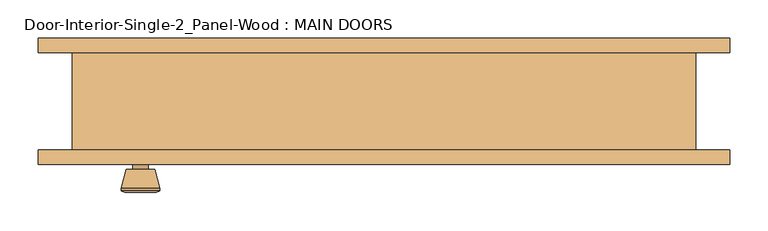
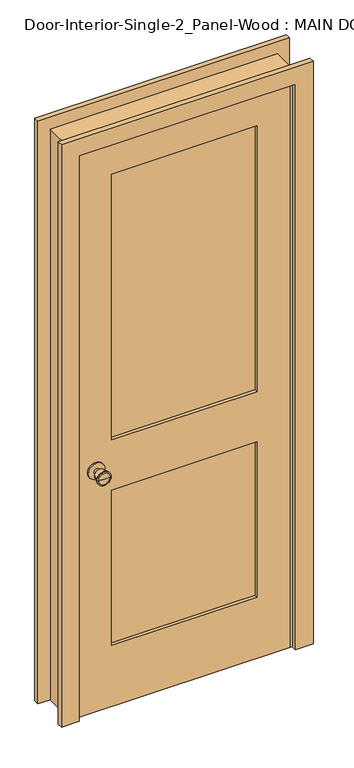
"""IFC4 building model written with IfcOpenShell, lengths in millimetres: door geometry, Door-Interior-Single-2_Panel-Wood : MAIN DOORS."""

from ifc_helpers import new_model, si_unit, point, frame, frame_2d, origin, place, context, project, spatial, polyline, circle_curve, trimmed, segment, composite_curve, outline, extrude, faceted_brep, source, transform, mapped, element, save
from ifc_brep_helpers import plane_surface, cylinder_surface, revolved_surface, advanced_brep


def door_interior_single_2_panel_wood_main_doors_4d656947(model_context):
    return source(origin(), model_context, "Body", "SolidModel", [
        advanced_brep(
        [(-317.5, -19.4, 914.4), (-327.5, -19.4, 914.4), (-307.5, -19.4, 914.4), (-297.0241324, 29.6, 914.4), (-337.9758676, 29.6, 914.4), (-317.5, 29.6, 914.4), (-292.5, 27.7721319, 914.4), (-342.5, 27.7721319, 914.4), (-292.5, 24.3084537, 914.4), (-342.5, 24.3084537, 914.4), (-298.863764, -0.4, 914.4), (-336.136236, -0.4, 914.4), (-307.5, -0.4, 914.4), (-327.5, -0.4, 914.4)],
        [
            (0, 1),
            (1, 2, circle_curve(frame((-317.5, -19.4, 914.4), z_axis=(0.0, -1.0, 0.0), x_axis=(-1.0, 0.0, 0.0)), 10.0)),
            (2, 0),
            (2, 1, circle_curve(frame((-317.5, -19.4, 914.4), z_axis=(0.0, -1.0, 0.0), x_axis=(-1.0, 0.0, 0.0)), 10.0)),
            (3, 4, circle_curve(frame((-317.5, 29.6, 914.4), z_axis=(0.0, 1.0, 0.0), x_axis=(-1.0, 0.0, 0.0)), 20.4758676)),
            (4, 5),
            (5, 3),
            (4, 3, circle_curve(frame((-317.5, 29.6, 914.4), z_axis=(0.0, 1.0, 0.0), x_axis=(-1.0, 0.0, 0.0)), 20.4758676)),
            (6, 7, circle_curve(frame((-317.5, 27.7721319, 914.4), z_axis=(0.0, 1.0, 0.0), x_axis=(-1.0, 0.0, 0.0)), 25.0)),
            (7, 4),
            (3, 6),
            (7, 6, circle_curve(frame((-317.5, 27.7721319, 914.4), z_axis=(0.0, 1.0, 0.0), x_axis=(-1.0, 0.0, 0.0)), 25.0)),
            (8, 9, circle_curve(frame((-317.5, 24.3084537, 914.4), z_axis=(0.0, 1.0, 0.0), x_axis=(-1.0, 0.0, 0.0)), 25.0)),
            (9, 7),
            (6, 8),
            (9, 8, circle_curve(frame((-317.5, 24.3084537, 914.4), z_axis=(0.0, 1.0, 0.0), x_axis=(-1.0, 0.0, 0.0)), 25.0)),
            (10, 11, circle_curve(frame((-317.5, -0.4, 914.4), z_axis=(0.0, 1.0, 0.0), x_axis=(-1.0, 0.0, 0.0)), 18.636236)),
            (11, 9),
            (8, 10),
            (11, 10, circle_curve(frame((-317.5, -0.4, 914.4), z_axis=(0.0, 1.0, 0.0), x_axis=(-1.0, 0.0, 0.0)), 18.636236)),
            (12, 13, circle_curve(frame((-317.5, -0.4, 914.4), z_axis=(0.0, 1.0, 0.0), x_axis=(-1.0, 0.0, 0.0)), 10.0)),
            (13, 11),
            (10, 12),
            (13, 12, circle_curve(frame((-317.5, -0.4, 914.4), z_axis=(0.0, 1.0, 0.0), x_axis=(-1.0, 0.0, 0.0)), 10.0)),
            (1, 13),
            (12, 2),
        ],
        [
            plane_surface(frame((-317.5, -19.4, 914.4), z_axis=(0.0, -1.0, 0.0), x_axis=(-1.0, 0.0, 0.0))),
            plane_surface(frame((-317.5, 29.6, 914.4), z_axis=(0.0, 1.0, 0.0), x_axis=(-1.0, 0.0, 0.0))),
            revolved_surface(polyline([(-337.9758676, 29.6, 914.4), (-342.5, 27.7721319, 914.4)]), (-317.5, -19.4, 914.4), (0.0, -1.0, 0.0)),
            cylinder_surface(frame((-317.5, -19.4, 914.4), z_axis=(0.0, -1.0, 0.0), x_axis=(-1.0, 0.0, 0.0)), 25.0),
            revolved_surface(polyline([(-342.5, 24.3084537, 914.4), (-336.136236, -0.4, 914.4)]), (-317.5, -19.4, 914.4), (0.0, -1.0, 0.0)),
            plane_surface(frame((-317.5, -0.4, 914.4), z_axis=(0.0, -1.0, 0.0), x_axis=(-1.0, 0.0, 0.0))),
            cylinder_surface(frame((-317.5, -19.4, 914.4), z_axis=(0.0, -1.0, 0.0), x_axis=(-1.0, 0.0, 0.0)), 10.0),
        ],
        [
            (0, [[1, 2, 3]]),
            (0, [[-3, 4, -1]]),
            (1, [[5, 6, 7]]),
            (1, [[8, -7, -6]]),
            (2, [[9, 10, -5, 11]]),
            (2, [[12, -11, -8, -10]]),
            (3, [[13, 14, -9, 15]]),
            (3, [[16, -15, -12, -14]]),
            (4, [[17, 18, -13, 19]]),
            (4, [[20, -19, -16, -18]]),
            (5, [[21, 22, -17, 23]]),
            (5, [[24, -23, -20, -22]]),
            (6, [[-2, 25, -21, 26]]),
            (6, [[-4, -26, -24, -25]]),
        ],
    ),
        extrude(outline(composite_curve([segment(trimmed(circle_curve(frame_2d((914.4, -317.5)), 30.0), [point((914.4, -347.5))], [point((914.4, -287.5))], False, "CARTESIAN"), True, "CONTINUOUS"), segment(trimmed(circle_curve(frame_2d((914.4, -317.5)), 30.0), [point((914.4, -287.5))], [point((914.4, -347.5))], False, "CARTESIAN"), True, "CONTINUOUS")], self_intersect=False)), frame((0.0, -25.4, 0.0), z_axis=(0.0, 1.0, 0.0), x_axis=(0.0, 0.0, 1.0)), (0.0, 0.0, 1.0), 6.0),
        advanced_brep(
        [(-317.5, -66.325, 914.4), (-307.5, -66.325, 914.4), (-327.5, -66.325, 914.4), (-297.0241324, -115.325, 914.4), (-317.5, -115.325, 914.4), (-337.9758676, -115.325, 914.4), (-292.5, -113.4971319, 914.4), (-342.5, -113.4971319, 914.4), (-292.5, -110.0334537, 914.4), (-342.5, -110.0334537, 914.4), (-298.863764, -85.325, 914.4), (-336.136236, -85.325, 914.4), (-307.5, -85.325, 914.4), (-327.5, -85.325, 914.4)],
        [
            (0, 1),
            (1, 2, circle_curve(frame((-317.5, -66.325, 914.4), z_axis=(0.0, 1.0, 0.0), x_axis=(-1.0, 0.0, 0.0)), 10.0)),
            (2, 0),
            (2, 1, circle_curve(frame((-317.5, -66.325, 914.4), z_axis=(0.0, 1.0, 0.0), x_axis=(-1.0, 0.0, 0.0)), 10.0)),
            (3, 4),
            (4, 5),
            (5, 3, circle_curve(frame((-317.5, -115.325, 914.4), z_axis=(0.0, -1.0, 0.0), x_axis=(-1.0, 0.0, 0.0)), 20.4758676)),
            (3, 5, circle_curve(frame((-317.5, -115.325, 914.4), z_axis=(0.0, -1.0, 0.0), x_axis=(-1.0, 0.0, 0.0)), 20.4758676)),
            (6, 3),
            (5, 7),
            (7, 6, circle_curve(frame((-317.5, -113.4971319, 914.4), z_axis=(0.0, -1.0, 0.0), x_axis=(-1.0, 0.0, 0.0)), 25.0)),
            (6, 7, circle_curve(frame((-317.5, -113.4971319, 914.4), z_axis=(0.0, -1.0, 0.0), x_axis=(-1.0, 0.0, 0.0)), 25.0)),
            (8, 6),
            (7, 9),
            (9, 8, circle_curve(frame((-317.5, -110.0334537, 914.4), z_axis=(0.0, -1.0, 0.0), x_axis=(-1.0, 0.0, 0.0)), 25.0)),
            (8, 9, circle_curve(frame((-317.5, -110.0334537, 914.4), z_axis=(0.0, -1.0, 0.0), x_axis=(-1.0, 0.0, 0.0)), 25.0)),
            (10, 8),
            (9, 11),
            (11, 10, circle_curve(frame((-317.5, -85.325, 914.4), z_axis=(0.0, -1.0, 0.0), x_axis=(-1.0, 0.0, 0.0)), 18.636236)),
            (10, 11, circle_curve(frame((-317.5, -85.325, 914.4), z_axis=(0.0, -1.0, 0.0), x_axis=(-1.0, 0.0, 0.0)), 18.636236)),
            (12, 10),
            (11, 13),
            (13, 12, circle_curve(frame((-317.5, -85.325, 914.4), z_axis=(0.0, -1.0, 0.0), x_axis=(-1.0, 0.0, 0.0)), 10.0)),
            (12, 13, circle_curve(frame((-317.5, -85.325, 914.4), z_axis=(0.0, -1.0, 0.0), x_axis=(-1.0, 0.0, 0.0)), 10.0)),
            (1, 12),
            (13, 2),
        ],
        [
            plane_surface(frame((-317.5, -66.325, 914.4), z_axis=(0.0, 1.0, 0.0), x_axis=(-1.0, 0.0, 0.0))),
            plane_surface(frame((-317.5, -115.325, 914.4), z_axis=(0.0, -1.0, 0.0), x_axis=(-1.0, 0.0, 0.0))),
            revolved_surface(polyline([(-337.9758676, -115.325, 914.4), (-342.5, -113.4971319, 914.4)]), (-317.5, -66.325, 914.4), (0.0, 1.0, 0.0)),
            cylinder_surface(frame((-317.5, -66.325, 914.4), z_axis=(0.0, 1.0, 0.0), x_axis=(-1.0, 0.0, 0.0)), 25.0),
            revolved_surface(polyline([(-342.5, -110.0334537, 914.4), (-336.136236, -85.325, 914.4)]), (-317.5, -66.325, 914.4), (0.0, 1.0, 0.0)),
            plane_surface(frame((-317.5, -85.325, 914.4), z_axis=(0.0, 1.0, 0.0), x_axis=(-1.0, 0.0, 0.0))),
            cylinder_surface(frame((-317.5, -66.325, 914.4), z_axis=(0.0, 1.0, 0.0), x_axis=(-1.0, 0.0, 0.0)), 10.0),
        ],
        [
            (0, [[1, 2, 3]]),
            (0, [[-3, 4, -1]]),
            (1, [[5, 6, 7]]),
            (1, [[-6, -5, 8]]),
            (2, [[9, -7, 10, 11]]),
            (2, [[-10, -8, -9, 12]]),
            (3, [[13, -11, 14, 15]]),
            (3, [[-14, -12, -13, 16]]),
            (4, [[17, -15, 18, 19]]),
            (4, [[-18, -16, -17, 20]]),
            (5, [[21, -19, 22, 23]]),
            (5, [[-22, -20, -21, 24]]),
            (6, [[25, -23, 26, -2]]),
            (6, [[-26, -24, -25, -4]]),
        ],
    ),
        extrude(outline(composite_curve([segment(trimmed(circle_curve(frame_2d((914.4, -317.5)), 30.0), [point((914.4, -347.5))], [point((914.4, -287.5))], False, "CARTESIAN"), True, "CONTINUOUS"), segment(trimmed(circle_curve(frame_2d((914.4, -317.5)), 30.0), [point((914.4, -287.5))], [point((914.4, -347.5))], False, "CARTESIAN"), True, "CONTINUOUS")], self_intersect=False)), frame((0.0, -66.325, 0.0), z_axis=(0.0, 1.0, 0.0), x_axis=(0.0, 0.0, 1.0)), (0.0, 0.0, 1.0), 6.0),
        faceted_brep([(406.4, -60.325, 0.0), (381.0, -60.325, 0.0), (381.0, -25.4, 0.0), (368.3, -25.4, 0.0), (368.3, 9.525, 0.0), (381.0, 9.525, 0.0), (381.0, 66.675, 0.0), (406.4, 66.675, 0.0), (406.4, 66.675, 2159.0), (406.4, -60.325, 2159.0), (381.0, 66.675, 2133.6), (-381.0, 66.675, 2133.6), (-381.0, 66.675, 0.0), (-406.4, 66.675, 0.0), (-406.4, 66.675, 2159.0), (381.0, 9.525, 2133.6), (368.3, 9.525, 2120.9), (-368.3, 9.525, 2120.9), (-368.3, 9.525, 0.0), (-381.0, 9.525, 0.0), (-381.0, 9.525, 2133.6), (368.3, -25.4, 2120.9), (381.0, -25.4, 2133.6), (-381.0, -25.4, 2133.6), (-381.0, -25.4, 0.0), (-368.3, -25.4, 0.0), (-368.3, -25.4, 2120.9), (381.0, -60.325, 2133.6), (-406.4, -60.325, 2159.0), (-406.4, -60.325, 0.0), (-381.0, -60.325, 0.0), (-381.0, -60.325, 2133.6)], [[[0, 1, 2, 3, 4, 5, 6, 7]], [[7, 8, 9, 0]], [[6, 10, 11, 12, 13, 14, 8, 7]], [[5, 15, 10, 6]], [[4, 16, 17, 18, 19, 20, 15, 5]], [[3, 21, 16, 4]], [[2, 22, 23, 24, 25, 26, 21, 3]], [[1, 27, 22, 2]], [[0, 9, 28, 29, 30, 31, 27, 1]], [[8, 14, 28, 9]], [[15, 20, 11, 10]], [[21, 26, 17, 16]], [[27, 31, 23, 22]], [[29, 13, 12, 19, 18, 25, 24, 30]], [[14, 13, 29, 28]], [[20, 19, 12, 11]], [[26, 25, 18, 17]], [[31, 30, 24, 23]]]),
        extrude(outline(polyline([(2133.6, -381.0), (0.0, -381.0), (0.0, 381.0), (2133.6, 381.0), (2133.6, -381.0)]), holes=[polyline([(2014.5375, -260.35), (2014.5375, 260.35), (1009.65, 260.35), (1009.65, -260.35), (2014.5375, -260.35)]), polyline([(819.15, -260.35), (819.15, 260.35), (231.775, 260.35), (231.775, -260.35), (819.15, -260.35)])]), frame((0.0, -60.325, 0.0), z_axis=(0.0, 1.0, 0.0), x_axis=(0.0, 0.0, 1.0)), (0.0, 0.0, 1.0), 34.925),
        extrude(outline(polyline([(260.35, -37.0416667), (260.35, -48.6833333), (-260.35, -48.6833333), (-260.35, -37.0416667), (260.35, -37.0416667)])), frame((0.0, 0.0, 1009.65), z_axis=(0.0, 0.0, 1.0), x_axis=(1.0, 0.0, 0.0)), (0.0, 0.0, 1.0), 1004.8875),
        extrude(outline(polyline([(260.35, -37.0416667), (260.35, -48.6833333), (-260.35, -48.6833333), (-260.35, -37.0416667), (260.35, -37.0416667)])), frame((0.0, 0.0, 231.775), z_axis=(0.0, 0.0, 1.0), x_axis=(1.0, 0.0, 0.0)), (0.0, 0.0, 1.0), 587.375),
        extrude(outline(polyline([(0.0, 450.85), (2203.45, 450.85), (2203.45, -450.85), (0.0, -450.85), (0.0, -387.35), (2139.95, -387.35), (2139.95, 387.35), (0.0, 387.35), (0.0, 450.85)])), frame((0.0, -79.375, 0.0), z_axis=(0.0, 1.0, 0.0), x_axis=(0.0, 0.0, 1.0)), (0.0, 0.0, 1.0), 19.05),
        extrude(outline(polyline([(0.0, 450.85), (2203.45, 450.85), (2203.45, -450.85), (0.0, -450.85), (0.0, -387.35), (2139.95, -387.35), (2139.95, 387.35), (0.0, 387.35), (0.0, 450.85)])), frame((0.0, 66.675, 0.0), z_axis=(0.0, 1.0, 0.0), x_axis=(0.0, 0.0, 1.0)), (0.0, 0.0, 1.0), 19.05),
    ])


if __name__ == "__main__":
    model = new_model("IFC4")
    model_context = context("Model", 3, world=origin())
    ifc_project = project(units=[si_unit("LENGTHUNIT", "METRE", prefix="MILLI")], contexts=[model_context])
    site = spatial("IfcSite", under=ifc_project)
    building = spatial("IfcBuilding", under=site)
    placement = place(None, origin())
    door_interior_single_2_panel_wood_main_doors_shape = door_interior_single_2_panel_wood_main_doors_4d656947(model_context)
    element("IfcDoor", 1, ObjectType="Door-Interior-Single-2_Panel-Wood : MAIN DOORS", at=placement, inside=building, context=model_context, shape_type="MappedRepresentation", body=[
        mapped(door_interior_single_2_panel_wood_main_doors_shape, transform((0.0, 0.0, 0.0), x_axis=(1.0, 0.0, 0.0), y_axis=(0.0, 1.0, 0.0), z_axis=(0.0, 0.0, 1.0))),
    ])
    save(model, "model.ifc")

# Revit data of these elements
# Type "Door-Interior-Single-2_Panel-Wood : MAIN DOORS"
#   Type Mark = "10"
#   Assembly Code = "C1020300"
#   Analytic Construction = "Wooden"
#   Top Rail = 0' - 4 11/16"
#   Thickness = 0' - 1 3/8"
#   Thermal Resistance (R) = 2.5876 (h·ft²·°F)/BTU
#   Swing Angle [instance default] = 90.00°
#   Stiles = 0' - 4 3/4"
#   Rough Width = 2' - 8"
#   Rough Height = 7' - 1"
#   Lock Rail = 0' - 7 1/2"
#   Height = 7' - 0"
#   Width = 2' - 6"
#   Heat Transfer Coefficient (U) = 0.3865 BTU/(h·ft²·°F)
#   Bottom Rail = 0' - 9 1/8"
#   Trim Material = Cherry
#   Panel Material = Cherry
#   Frame Material = Cherry
#   Door Handle Material = Aluminum
#   Visual Light Transmittance = 0
#   Solar Heat Gain Coefficient = 0
#   Wall Closure = (empty or 0)
#   Function = (empty or 0)
# Element 1 (IfcDoor, "Door-Interior-Single-2_Panel-Wood : MAIN DOORS")
#   Materials on its faces: "Cherry", "Aluminum"
# Materials
#   "Cherry": class "Wood", colour RGB 226 177 128, transparency 0, Description = "Prunus Serotina", Cost = 0
#   "Aluminum": class "Metal", colour RGB 247 247 247, transparency 0, Description = "Aluminum 6061", Cost = 0
